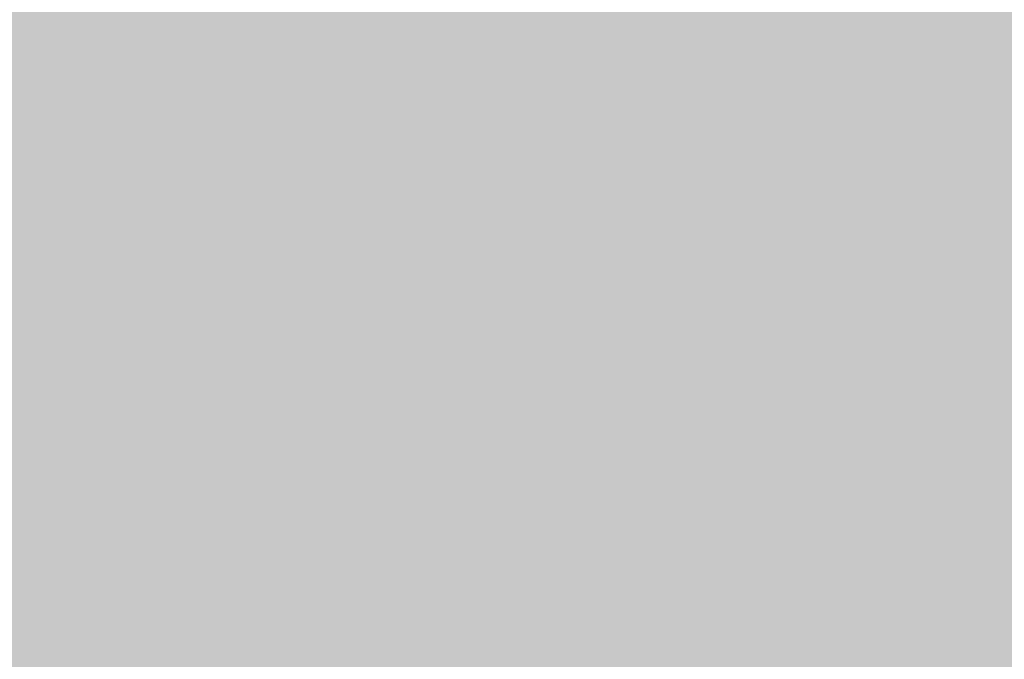
# Model space of a CAD drawing. Units: millimetres. Extents: x 0 to 2267, y 0 to 1823.
# Tile 133 of 256: x 1590 to 1632, y 1243 to 1271. Entities that reach past the tile are written whole.
import ezdxf

# ---------------------------------------------------------------- set-up
doc = ezdxf.new("R2010")
doc.units = ezdxf.units.MM
doc.header["$MEASUREMENT"] = 0
doc.layers.add('M-DIMS', color=2, linetype='Continuous', lineweight=25)
doc.layers.add('M-HATC', color=252, linetype='Continuous', lineweight=18)
doc.styles.get("Standard").update_dxf_attribs({"font": 'arial.ttf'})
doc.dimstyles.get("Standard").update_dxf_attribs({"dimtxt": 7, "dimasz": 4, "dimexe": 0.18, "dimexo": 0.0625, "dimgap": 0.09, "dimtad": 0, "dimdec": 0, "dimzin": 0, "dimdsep": 46, "dimtxsty": 'Standard', "dimcen": 0.09, "dimadec": 0, "dimazin": 0, "dimtfac": 1, "dimtdec": 0, "dimtofl": 0, "dimtmove": 0, "dimatfit": 3, "dimfxl": 1, "dimtolj": 1, "dimtzin": 0, "dimarcsym": 0})

# ---------------------------------------------------------------- blocks, each defined once
blk = doc.blocks.new('*D19')
at = {"layer": 'Defpoints', "color": 0, "transparency": 16777216}
for p in [(1605.34, 1483.304), (1445.529, 1333.885)]:
    blk.add_point(p, dxfattribs=at)
at = {"layer": 'M-DIMS', "color": 0, "lineweight": -2, "transparency": 16777216}
for p, q in [((1605.25, 1483.304), (1605.43, 1483.304)), ((1605.34, 1483.214), (1605.34, 1483.394)), ((1366.324, 1259.831), (1442.607, 1331.153))]:
    blk.add_line(p, q, dxfattribs=at)
at = {"layer": 'M-DIMS', "color": 0, "transparency": 16777216}
blk.add_solid([(1442.152, 1331.64), (1443.063, 1330.666), (1445.529, 1333.885)], dxfattribs=at)
at = {"layer": 'M-DIMS', "color": 0, "transparency": 16777216, "insert": (1349.643, 1244.233), "char_height": 7, "attachment_point": 5, "rotation": 43.0753}
blk.add_mtext('\\A1;2X R218.8', dxfattribs=at)

msp = doc.modelspace()

# ---------------------------------------------------------------- hatches: boundary and pattern name
at = {"layer": 'M-HATC'}
h = msp.add_hatch(color=256, dxfattribs=at)
h.dxf.hatch_style = 1
h.paths.add_polyline_path([(2065.771, 1618.062, 0.236068), (2055.771, 1638.062), (1381.087, 1638.062, 0.236068), (1371.087, 1618.062), (1371.087, 1603.062), (2055.771, 1603.062), (2065.771, 1603.062)])
h.paths.add_polyline_path([(2062.772, 1550.296), (2062.772, 1560.296), (1374.086, 1560.296), (1374.086, 1550.296), (1374.086, 1540.296), (1384.086, 1540.296), (1389.086, 1540.296), (2062.772, 1540.296)])
h.paths.add_polyline_path([(1930.929, 1282.766), (1505.929, 1282.766), (1587.628, 1235.597, 0.131652), (1600.128, 1232.247), (1836.73, 1232.247, 0.131652), (1849.23, 1235.597)])
h.paths.add_polyline_path([(1930.929, 1117.417), (1905.929, 1117.417), (1505.929, 1117.417), (1505.929, 1077.417), (1930.929, 1077.417)])
h = msp.add_hatch(color=256, dxfattribs=at)
h.dxf.hatch_style = 1
h.paths.add_polyline_path([(2055.771, 1603.062), (1381.087, 1603.062), (1381.087, 1598.062), (2055.771, 1598.062)])
h.paths.add_polyline_path([(2055.771, 1598.062), (1381.087, 1598.062), (1381.087, 1593.062), (2055.771, 1593.062)])
h.paths.add_polyline_path([(2051.307, 1536.761), (1385.55, 1536.761), (1385.55, 1526.761), (1387.55, 1526.761), (1388.537, 1525.053), (1385.332, 1521.233), (1385.332, 1521.223), (2050.254, 1522.749), (2048.321, 1525.053), (2049.307, 1526.761), (2051.307, 1526.761)])
edge = h.paths.add_edge_path()
edge.add_arc((1847.535, 1379.149), 135, 222.60306, 222.89085, ccw=False)
edge.add_line((1748.166, 1287.766), (1683.092, 1287.766))
edge.add_arc((1583.724, 1379.149), 135, 317.10915, 317.39694, ccw=False)
edge.add_arc((1678.969, 1290.671), 5, 222.8909, 317.1091, ccw=False)
edge.add_arc((1774.213, 1379.149), 135, 222.60306, 222.89085, ccw=False)
edge.add_line((1674.845, 1287.766), (1609.771, 1287.766))
edge.add_arc((1510.403, 1379.149), 135, 317.10915, 317.39694, ccw=False)
edge.add_arc((1605.647, 1290.671), 5, 222.8909, 317.1091, ccw=False)
edge.add_arc((1700.892, 1379.149), 135, 222.60306, 222.89085, ccw=False)
edge.add_line((1601.524, 1287.766), (1536.45, 1287.766))
edge.add_arc((1437.081, 1379.149), 135, 317.10915, 317.39694, ccw=False)
edge.add_arc((1532.326, 1290.671), 5, 222.8909, 317.1091, ccw=False)
edge.add_arc((1627.571, 1379.149), 135, 222.60306, 222.89085, ccw=False)
edge.add_line((1528.203, 1287.766), (1505.929, 1287.766))
edge.add_spline(control_points=[(1505.929, 1287.766), (1504.262, 1287.766), (1504.262, 1282.766), (1505.929, 1282.766)], knot_values=[0, 0, 0, 0, 5, 5, 5, 5], degree=3, periodic=0)
edge.add_line((1505.929, 1282.766), (1930.929, 1282.766))
edge.add_spline(control_points=[(1930.929, 1282.766), (1932.596, 1282.766), (1932.596, 1287.766), (1930.929, 1287.766)], knot_values=[0, 0, 0, 0, 5, 5, 5, 5], degree=3, periodic=0)
edge.add_line((1930.929, 1287.766), (1903.056, 1287.766))
edge.add_arc((1803.688, 1379.149), 135, 317.10915, 317.39694, ccw=False)
edge.add_arc((1898.932, 1290.671), 5, 222.8909, 317.1091, ccw=False)
edge.add_arc((1994.177, 1379.149), 135, 222.60306, 222.89085, ccw=False)
edge.add_line((1894.809, 1287.766), (1829.735, 1287.766))
edge.add_arc((1730.366, 1379.149), 135, 317.10915, 317.39694, ccw=False)
edge.add_arc((1825.611, 1290.671), 5, 222.8909, 317.1091, ccw=False)
edge.add_arc((1920.856, 1379.149), 135, 222.60306, 222.89085, ccw=False)
edge.add_line((1821.487, 1287.766), (1756.413, 1287.766))
edge.add_arc((1657.045, 1379.149), 135, 317.10915, 317.39694, ccw=False)
edge.add_arc((1752.29, 1290.671), 5, 222.8909, 317.1091, ccw=False)
edge = h.paths.add_edge_path()
edge.add_spline(control_points=[(1843.429, 1227.247), (1845.096, 1227.247), (1845.096, 1232.247), (1843.429, 1232.247)], knot_values=[0, 0, 0, 0, 5, 5, 5, 5], degree=3, periodic=0)
edge.add_line((1843.429, 1232.247), (1593.429, 1232.247))
edge.add_spline(control_points=[(1593.429, 1232.247), (1591.762, 1232.247), (1591.762, 1227.247), (1593.429, 1227.247)], knot_values=[0, 0, 0, 0, 5, 5, 5, 5], degree=3, periodic=0)
edge.add_line((1593.429, 1227.247), (1843.429, 1227.247))
h.paths.add_polyline_path([(1905.929, 1127.417), (1530.929, 1127.417, 0.414214), (1520.929, 1117.417), (1530.929, 1117.417), (1915.929, 1117.417, 0.414214)])
edge = h.paths.add_edge_path()
edge.add_arc((1397.086, 1498.408), 12.73, 90.7821, 190.8787, ccw=False)
edge.add_line((1396.912, 1511.136), (1428.01, 1511.349))
edge.add_line((1428.01, 1511.349), (1433.01, 1511.349))
edge.add_line((1433.01, 1511.349), (1434.439, 1511.349))
edge.add_arc((1419.474, 1498.08), 20, 41.561, 74.0821)
edge.add_line((1424.959, 1517.314), (1399.935, 1517.256))
edge.add_spline(control_points=[(1399.931, 1517.256), (1399.884, 1517.213), (1399.833, 1517.169), (1399.777, 1517.124)], knot_values=[11.567499, 11.567499, 11.567499, 11.567499, 11.814249, 11.814249, 11.814249, 11.814249], degree=3, periodic=0)
edge.add_spline(control_points=[(1399.633, 1517.01), (1399.583, 1516.972), (1399.531, 1516.934), (1399.476, 1516.895)], knot_values=[11.167718, 11.167718, 11.167718, 11.167718, 11.365188, 11.365188, 11.365188, 11.365188], degree=3, periodic=0)
edge.add_spline(control_points=[(1399.34, 1516.8), (1399.151, 1516.672), (1398.938, 1516.538), (1398.704, 1516.399)], knot_values=[10.376405, 10.376405, 10.376405, 10.376405, 11.00994, 11.00994, 11.00994, 11.00994], degree=3, periodic=0)
edge.add_spline(control_points=[(1398.657, 1516.372), (1398.579, 1516.326), (1398.498, 1516.28), (1398.415, 1516.233)], knot_values=[10.125175, 10.125175, 10.125175, 10.125175, 10.334406, 10.334406, 10.334406, 10.334406], degree=3, periodic=0)
edge.add_spline(control_points=[(1398.264, 1516.149), (1398.196, 1516.111), (1398.126, 1516.073), (1398.055, 1516.035)], knot_values=[9.832246, 9.832246, 9.832246, 9.832246, 9.999658, 9.999658, 9.999658, 9.999658], degree=3, periodic=0)
edge.add_spline(control_points=[(1397.999, 1516.005), (1397.731, 1515.862), (1397.446, 1515.717), (1397.147, 1515.571)], knot_values=[9.161808, 9.161808, 9.161808, 9.161808, 9.787769, 9.787769, 9.787769, 9.787769], degree=3, periodic=0)
edge.add_spline(control_points=[(1397.147, 1515.571), (1396.842, 1515.423), (1396.522, 1515.274), (1396.191, 1515.126)], knot_values=[8.524455, 8.524455, 8.524455, 8.524455, 9.161808, 9.161808, 9.161808, 9.161808], degree=3, periodic=0)
edge.add_spline(control_points=[(1396.078, 1515.076), (1395.985, 1515.035), (1395.892, 1514.994), (1395.798, 1514.953)], knot_values=[8.275193, 8.275193, 8.275193, 8.275193, 8.451726, 8.451726, 8.451726, 8.451726], degree=3, periodic=0)
edge.add_spline(control_points=[(1395.602, 1514.869), (1395.5, 1514.826), (1395.397, 1514.782), (1395.293, 1514.739)], knot_values=[7.962917, 7.962917, 7.962917, 7.962917, 8.152764, 8.152764, 8.152764, 8.152764], degree=3, periodic=0)
edge.add_spline(control_points=[(1395.212, 1514.706), (1394.828, 1514.547), (1394.435, 1514.393), (1394.036, 1514.244)], knot_values=[7.21254, 7.21254, 7.21254, 7.21254, 7.913148, 7.913148, 7.913148, 7.913148], degree=3, periodic=0)
edge.add_spline(control_points=[(1394.036, 1514.244), (1393.708, 1514.121), (1393.375, 1514.003), (1393.043, 1513.889)], knot_values=[6.633733, 6.633733, 6.633733, 6.633733, 7.21254, 7.21254, 7.21254, 7.21254], degree=3, periodic=0)
edge.add_spline(control_points=[(1392.821, 1513.815), (1392.72, 1513.781), (1392.618, 1513.748), (1392.517, 1513.715)], knot_values=[6.328796, 6.328796, 6.328796, 6.328796, 6.505493, 6.505493, 6.505493, 6.505493], degree=3, periodic=0)
edge.add_spline(control_points=[(1392.517, 1513.715), (1392.319, 1513.652), (1392.121, 1513.59), (1391.924, 1513.531)], knot_values=[5.984605, 5.984605, 5.984605, 5.984605, 6.328796, 6.328796, 6.328796, 6.328796], degree=3, periodic=0)
edge.add_spline(control_points=[(1391.792, 1513.491), (1391.312, 1513.35), (1390.838, 1513.224), (1390.378, 1513.117)], knot_values=[5.066697, 5.066697, 5.066697, 5.066697, 5.907055, 5.907055, 5.907055, 5.907055], degree=3, periodic=0)
edge.add_spline(control_points=[(1390.378, 1513.117), (1390.18, 1513.071), (1389.984, 1513.028), (1389.791, 1512.99)], knot_values=[4.70367, 4.70367, 4.70367, 4.70367, 5.066695, 5.066695, 5.066695, 5.066695], degree=3, periodic=0)
edge.add_spline(control_points=[(1389.422, 1512.92), (1389.246, 1512.889), (1389.073, 1512.862), (1388.904, 1512.838)], knot_values=[4.130571, 4.130571, 4.130571, 4.130571, 4.469816, 4.469816, 4.469816, 4.469816], degree=3, periodic=0)
edge.add_spline(control_points=[(1388.904, 1512.838), (1388.591, 1512.795), (1388.291, 1512.764), (1388.007, 1512.749)], knot_values=[3.504031, 3.504031, 3.504031, 3.504031, 4.130571, 4.130571, 4.130571, 4.130571], degree=3, periodic=0)
edge.add_spline(control_points=[(1387.936, 1512.746), (1387.854, 1512.742), (1387.773, 1512.74), (1387.694, 1512.739)], knot_values=[3.268866, 3.268866, 3.268866, 3.268866, 3.451164, 3.451164, 3.451164, 3.451164], degree=3, periodic=0)
edge.add_spline(control_points=[(1387.335, 1512.744), (1387.208, 1512.75), (1387.085, 1512.76), (1386.967, 1512.774)], knot_values=[2.670686, 2.670686, 2.670686, 2.670686, 2.984, 2.984, 2.984, 2.984], degree=3, periodic=0)
edge.add_spline(control_points=[(1386.833, 1512.792), (1386.821, 1512.794), (1386.809, 1512.796), (1386.797, 1512.798)], knot_values=[2.516981, 2.516981, 2.516981, 2.516981, 2.549528, 2.549528, 2.549528, 2.549528], degree=3, periodic=0)
edge.add_spline(control_points=[(1386.453, 1512.873), (1386.426, 1512.881), (1386.399, 1512.889), (1386.373, 1512.897)], knot_values=[2.095869, 2.095869, 2.095869, 2.095869, 2.17941, 2.17941, 2.17941, 2.17941], degree=3, periodic=0)
edge.add_spline(control_points=[(1386.069, 1513.019), (1386.063, 1513.022), (1386.058, 1513.025), (1386.052, 1513.028)], knot_values=[1.72453, 1.72453, 1.72453, 1.72453, 1.745933, 1.745933, 1.745933, 1.745933], degree=3, periodic=0)
edge.add_arc((1399.474, 1498.08), 20, 131.8243, 180)
edge.add_arc((1630.334, 1505.548), 250.971, 181.70518, 236.42798)
edge.add_arc((1605.34, 1483.304), 218.782, 238.66083, 243.34961)
edge.add_arc((1647.091, 1510.359), 262.899, 183.12984, 237.85344, ccw=False)
h.paths.add_polyline_path([(1406.537, 1391.964, 0.149382), (1491.551, 1296.442, -0.129517)], flags=17)
edge = h.paths.add_edge_path()
edge.add_arc((2037.384, 1498.08), 20, 0, 48.2659)
edge.add_spline(control_points=[(2050.697, 1513.005), (2050.651, 1512.985), (2050.603, 1512.966), (2050.554, 1512.948)], knot_values=[1.835652, 1.835652, 1.835652, 1.835652, 2.000781, 2.000781, 2.000781, 2.000781], degree=3, periodic=0)
edge.add_spline(control_points=[(2050.462, 1512.917), (2050.479, 1512.922), (2050.496, 1512.928), (2050.513, 1512.934)], knot_values=[2.045477, 2.045477, 2.045477, 2.045477, 2.101389, 2.101389, 2.101389, 2.101389], degree=3, periodic=0)
edge.add_spline(control_points=[(2050.129, 1512.834), (2050.198, 1512.847), (2050.266, 1512.862), (2050.331, 1512.879)], knot_values=[2.237629, 2.237629, 2.237629, 2.237629, 2.435841, 2.435841, 2.435841, 2.435841], degree=3, periodic=0)
edge.add_spline(control_points=[(2050.095, 1512.828), (2050.106, 1512.83), (2050.118, 1512.832), (2050.129, 1512.834)], knot_values=[2.435841, 2.435841, 2.435841, 2.435841, 2.468321, 2.468321, 2.468321, 2.468321], degree=3, periodic=0)
edge.add_spline(control_points=[(2049.784, 1512.785), (2049.855, 1512.792), (2049.924, 1512.801), (2049.992, 1512.811)], knot_values=[2.563852, 2.563852, 2.563852, 2.563852, 2.748541, 2.748541, 2.748541, 2.748541], degree=3, periodic=0)
edge.add_spline(control_points=[(2049.405, 1512.762), (2049.536, 1512.765), (2049.663, 1512.773), (2049.784, 1512.785)], knot_values=[2.748541, 2.748541, 2.748541, 2.748541, 3.064882, 3.064882, 3.064882, 3.064882], degree=3, periodic=0)
edge.add_spline(control_points=[(2049.17, 1512.76), (2049.234, 1512.759), (2049.297, 1512.759), (2049.358, 1512.761)], knot_values=[3.102309, 3.102309, 3.102309, 3.102309, 3.2503, 3.2503, 3.2503, 3.2503], degree=3, periodic=0)
edge.add_spline(control_points=[(2048.857, 1512.769), (2048.964, 1512.764), (2049.068, 1512.761), (2049.17, 1512.76)], knot_values=[3.2503, 3.2503, 3.2503, 3.2503, 3.486069, 3.486069, 3.486069, 3.486069], degree=3, periodic=0)
edge.add_spline(control_points=[(2048.692, 1512.779), (2048.373, 1512.801), (2048.035, 1512.841), (2047.682, 1512.897)], knot_values=[3.606429, 3.606429, 3.606429, 3.606429, 4.2989, 4.2989, 4.2989, 4.2989], degree=3, periodic=0)
edge.add_spline(control_points=[(2047.682, 1512.897), (2047.546, 1512.919), (2047.408, 1512.942), (2047.268, 1512.969)], knot_values=[4.2989, 4.2989, 4.2989, 4.2989, 4.565769, 4.565769, 4.565769, 4.565769], degree=3, periodic=0)
edge.add_spline(control_points=[(2047.268, 1512.969), (2047.145, 1512.991), (2047.021, 1513.016), (2046.895, 1513.042)], knot_values=[4.565769, 4.565769, 4.565769, 4.565769, 4.799971, 4.799971, 4.799971, 4.799971], degree=3, periodic=0)
edge.add_spline(control_points=[(2046.895, 1513.042), (2046.529, 1513.119), (2046.151, 1513.209), (2045.768, 1513.311)], knot_values=[4.799971, 4.799971, 4.799971, 4.799971, 5.483718, 5.483718, 5.483718, 5.483718], degree=3, periodic=0)
edge.add_spline(control_points=[(2045.768, 1513.311), (2045.372, 1513.415), (2044.97, 1513.532), (2044.566, 1513.659)], knot_values=[5.483718, 5.483718, 5.483718, 5.483718, 6.187866, 6.187866, 6.187866, 6.187866], degree=3, periodic=0)
edge.add_spline(control_points=[(2044.566, 1513.659), (2044.415, 1513.706), (2044.263, 1513.755), (2044.112, 1513.805)], knot_values=[6.187866, 6.187866, 6.187866, 6.187866, 6.451551, 6.451551, 6.451551, 6.451551], degree=3, periodic=0)
edge.add_spline(control_points=[(2044.112, 1513.805), (2043.997, 1513.843), (2043.882, 1513.881), (2043.767, 1513.92)], knot_values=[6.451551, 6.451551, 6.451551, 6.451551, 6.651434, 6.651434, 6.651434, 6.651434], degree=3, periodic=0)
edge.add_spline(control_points=[(2043.767, 1513.92), (2043.372, 1514.055), (2042.977, 1514.198), (2042.589, 1514.346)], knot_values=[6.651434, 6.651434, 6.651434, 6.651434, 7.338879, 7.338879, 7.338879, 7.338879], degree=3, periodic=0)
edge.add_spline(control_points=[(2042.589, 1514.346), (2042.164, 1514.507), (2041.746, 1514.675), (2041.341, 1514.846)], knot_values=[7.338879, 7.338879, 7.338879, 7.338879, 8.089209, 8.089209, 8.089209, 8.089209], degree=3, periodic=0)
edge.add_spline(control_points=[(2041.341, 1514.846), (2041.103, 1514.946), (2040.869, 1515.048), (2040.64, 1515.15)], knot_values=[8.089209, 8.089209, 8.089209, 8.089209, 8.529587, 8.529587, 8.529587, 8.529587], degree=3, periodic=0)
edge.add_spline(control_points=[(2040.51, 1515.209), (2040.082, 1515.402), (2039.675, 1515.597), (2039.295, 1515.789)], knot_values=[8.613818, 8.613818, 8.613818, 8.613818, 9.44571, 9.44571, 9.44571, 9.44571], degree=3, periodic=0)
edge.add_spline(control_points=[(2039.295, 1515.789), (2039.062, 1515.907), (2038.839, 1516.025), (2038.629, 1516.14)], knot_values=[9.44571, 9.44571, 9.44571, 9.44571, 9.956404, 9.956404, 9.956404, 9.956404], degree=3, periodic=0)
edge.add_spline(control_points=[(2038.629, 1516.14), (2038.519, 1516.2), (2038.412, 1516.26), (2038.309, 1516.319)], knot_values=[9.956404, 9.956404, 9.956404, 9.956404, 10.223542, 10.223542, 10.223542, 10.223542], degree=3, periodic=0)
edge.add_spline(control_points=[(2038.309, 1516.319), (2038.214, 1516.374), (2038.122, 1516.428), (2038.033, 1516.481)], knot_values=[10.223542, 10.223542, 10.223542, 10.223542, 10.47051, 10.47051, 10.47051, 10.47051], degree=3, periodic=0)
edge.add_spline(control_points=[(2038.033, 1516.481), (2037.786, 1516.63), (2037.564, 1516.773), (2037.372, 1516.909)], knot_values=[10.47051, 10.47051, 10.47051, 10.47051, 11.15767, 11.15767, 11.15767, 11.15767], degree=3, periodic=0)
edge.add_spline(control_points=[(2037.372, 1516.909), (2037.279, 1516.975), (2037.193, 1517.04), (2037.114, 1517.102)], knot_values=[11.15767, 11.15767, 11.15767, 11.15767, 11.49227, 11.49227, 11.49227, 11.49227], degree=3, periodic=0)
edge.add_spline(control_points=[(2036.856, 1517.326), (2036.915, 1517.269), (2036.981, 1517.21), (2037.056, 1517.149)], knot_values=[11.577341, 11.577341, 11.577341, 11.577341, 11.91035, 11.91035, 11.91035, 11.91035], degree=3, periodic=0)
edge.add_spline(control_points=[(2036.807, 1517.375), (2036.823, 1517.359), (2036.839, 1517.342), (2036.856, 1517.326)], knot_values=[11.91035, 11.91035, 11.91035, 11.91035, 12.007402, 12.007402, 12.007402, 12.007402], degree=3, periodic=0)
edge.add_spline(control_points=[(2036.702, 1517.494), (2036.71, 1517.483), (2036.72, 1517.472), (2036.729, 1517.461)], knot_values=[12.184155, 12.184155, 12.184155, 12.184155, 12.255409, 12.255409, 12.255409, 12.255409], degree=3, periodic=0)
edge.add_spline(control_points=[(2036.616, 1517.621), (2036.62, 1517.613), (2036.624, 1517.606), (2036.629, 1517.598)], knot_values=[12.487913, 12.487913, 12.487913, 12.487913, 12.541035, 12.541035, 12.541035, 12.541035], degree=3, periodic=0)
edge.add_spline(control_points=[(2036.563, 1517.786), (2036.564, 1517.779), (2036.564, 1517.773), (2036.565, 1517.766)], knot_values=[12.911761, 12.911761, 12.911761, 12.911761, 12.968286, 12.968286, 12.968286, 12.968286], degree=3, periodic=0)
edge.add_spline(control_points=[(2036.617, 1517.93), (2036.612, 1517.926), (2036.609, 1517.921), (2036.605, 1517.916)], knot_values=[13.382527, 13.382527, 13.382527, 13.382527, 13.433791, 13.433791, 13.433791, 13.433791], degree=3, periodic=0)
edge.add_spline(control_points=[(2036.749, 1518.017), (2036.736, 1518.012), (2036.724, 1518.006), (2036.712, 1518)], knot_values=[13.726299, 13.726299, 13.726299, 13.726299, 13.809928, 13.809928, 13.809928, 13.809928], degree=3, periodic=0)
edge.add_spline(control_points=[(2036.86, 1518.053), (2036.839, 1518.047), (2036.818, 1518.042), (2036.799, 1518.035)], knot_values=[13.910887, 13.910887, 13.910887, 13.910887, 14.02153, 14.02153, 14.02153, 14.02153], degree=3, periodic=0)
edge.add_line((2036.964, 1518.08), (2032.384, 1518.08))
edge.add_line((2032.384, 1518.08), (2027.384, 1518.08))
edge.add_line((2027.384, 1518.08), (2022.384, 1518.08))
edge.add_line((2022.384, 1518.08), (2017.384, 1518.08))
edge.add_arc((2017.384, 1498.08), 20, 90, 138.439)
edge.add_line((2002.419, 1511.349), (2003.848, 1511.349))
edge.add_line((2003.848, 1511.349), (2008.848, 1511.349))
edge.add_line((2008.848, 1511.349), (2039.772, 1511.138))
edge.add_arc((2039.772, 1498.408), 12.73, -10.8787, 90, ccw=False)
edge.add_arc((1789.767, 1510.359), 262.899, 302.14656, 356.87016, ccw=False)
edge.add_arc((1831.518, 1483.304), 218.782, 296.65039, 301.33917)
edge.add_arc((1806.524, 1505.548), 250.971, 303.57202, 358.29482)
h.paths.add_polyline_path([(2030.321, 1391.964, -0.129517), (1945.307, 1296.442, 0.149382)], flags=17)
edge = h.paths.add_edge_path()
edge.add_spline(control_points=[(2037.246, 1518.082), (2037.29, 1518.081), (2037.336, 1518.08), (2037.384, 1518.08)], knot_values=[0.000012, 0.000012, 0.000012, 0.000012, 0.144754, 0.144754, 0.144754, 0.144754], degree=3, periodic=0)
edge.add_line((2037.336, 1518.08), (2037.01, 1518.08))
edge.add_spline(control_points=[(2037.01, 1518.08), (2036.982, 1518.077), (2036.956, 1518.073), (2036.931, 1518.068)], knot_values=[14.13465, 14.13465, 14.13465, 14.13465, 14.247197, 14.247197, 14.247197, 14.247197], degree=3, periodic=0)
edge.add_spline(control_points=[(2036.931, 1518.068), (2036.928, 1518.067), (2036.924, 1518.067), (2036.921, 1518.066)], knot_values=[14.118315, 14.118315, 14.118315, 14.118315, 14.13465, 14.13465, 14.13465, 14.13465], degree=3, periodic=0)
edge.add_spline(control_points=[(2036.921, 1518.066), (2036.912, 1518.064), (2036.903, 1518.063), (2036.895, 1518.061)], knot_values=[14.078086, 14.078086, 14.078086, 14.078086, 14.118315, 14.118315, 14.118315, 14.118315], degree=3, periodic=0)
edge.add_spline(control_points=[(2036.895, 1518.061), (2036.883, 1518.058), (2036.872, 1518.056), (2036.86, 1518.053)], knot_values=[14.02153, 14.02153, 14.02153, 14.02153, 14.078086, 14.078086, 14.078086, 14.078086], degree=3, periodic=0)
edge.add_spline(control_points=[(2036.86, 1518.053), (2036.839, 1518.047), (2036.818, 1518.042), (2036.799, 1518.035)], knot_values=[13.910887, 13.910887, 13.910887, 13.910887, 14.02153, 14.02153, 14.02153, 14.02153], degree=3, periodic=0)
edge.add_spline(control_points=[(2036.799, 1518.035), (2036.798, 1518.035), (2036.797, 1518.035), (2036.797, 1518.035)], knot_values=[13.906906, 13.906906, 13.906906, 13.906906, 13.910887, 13.910887, 13.910887, 13.910887], degree=3, periodic=0)
edge.add_spline(control_points=[(2036.797, 1518.035), (2036.788, 1518.032), (2036.78, 1518.029), (2036.772, 1518.026)], knot_values=[13.857826, 13.857826, 13.857826, 13.857826, 13.906906, 13.906906, 13.906906, 13.906906], degree=3, periodic=0)
edge.add_spline(control_points=[(2036.772, 1518.026), (2036.764, 1518.023), (2036.756, 1518.02), (2036.749, 1518.017)], knot_values=[13.809928, 13.809928, 13.809928, 13.809928, 13.857826, 13.857826, 13.857826, 13.857826], degree=3, periodic=0)
edge.add_spline(control_points=[(2036.749, 1518.017), (2036.736, 1518.012), (2036.724, 1518.006), (2036.712, 1518)], knot_values=[13.726299, 13.726299, 13.726299, 13.726299, 13.809928, 13.809928, 13.809928, 13.809928], degree=3, periodic=0)
edge.add_spline(control_points=[(2036.712, 1518), (2036.712, 1518), (2036.712, 1518), (2036.711, 1518)], knot_values=[13.723993, 13.723993, 13.723993, 13.723993, 13.726299, 13.726299, 13.726299, 13.726299], degree=3, periodic=0)
edge.add_spline(control_points=[(2036.711, 1518), (2036.706, 1517.997), (2036.701, 1517.994), (2036.696, 1517.992)], knot_values=[13.686536, 13.686536, 13.686536, 13.686536, 13.723993, 13.723993, 13.723993, 13.723993], degree=3, periodic=0)
edge.add_spline(control_points=[(2036.696, 1517.992), (2036.692, 1517.989), (2036.687, 1517.987), (2036.683, 1517.984)], knot_values=[13.651251, 13.651251, 13.651251, 13.651251, 13.686536, 13.686536, 13.686536, 13.686536], degree=3, periodic=0)
edge.add_spline(control_points=[(2036.683, 1517.984), (2036.676, 1517.98), (2036.67, 1517.976), (2036.664, 1517.971)], knot_values=[13.596804, 13.596804, 13.596804, 13.596804, 13.651251, 13.651251, 13.651251, 13.651251], degree=3, periodic=0)
edge.add_spline(control_points=[(2036.664, 1517.971), (2036.664, 1517.971), (2036.663, 1517.971), (2036.663, 1517.971)], knot_values=[13.593956, 13.593956, 13.593956, 13.593956, 13.596804, 13.596804, 13.596804, 13.596804], degree=3, periodic=0)
edge.add_spline(control_points=[(2036.663, 1517.971), (2036.66, 1517.969), (2036.658, 1517.967), (2036.655, 1517.965)], knot_values=[13.570322, 13.570322, 13.570322, 13.570322, 13.593956, 13.593956, 13.593956, 13.593956], degree=3, periodic=0)
edge.add_spline(control_points=[(2036.655, 1517.965), (2036.653, 1517.963), (2036.65, 1517.961), (2036.647, 1517.959)], knot_values=[13.545477, 13.545477, 13.545477, 13.545477, 13.570322, 13.570322, 13.570322, 13.570322], degree=3, periodic=0)
edge.add_spline(control_points=[(2036.647, 1517.959), (2036.647, 1517.959), (2036.647, 1517.959), (2036.647, 1517.959)], knot_values=[13.543931, 13.543931, 13.543931, 13.543931, 13.545477, 13.545477, 13.545477, 13.545477], degree=3, periodic=0)
edge.add_spline(control_points=[(2036.647, 1517.959), (2036.641, 1517.954), (2036.636, 1517.949), (2036.631, 1517.945)], knot_values=[13.488237, 13.488237, 13.488237, 13.488237, 13.543931, 13.543931, 13.543931, 13.543931], degree=3, periodic=0)
edge.add_spline(control_points=[(2036.631, 1517.945), (2036.628, 1517.942), (2036.626, 1517.94), (2036.623, 1517.937)], knot_values=[13.460307, 13.460307, 13.460307, 13.460307, 13.488237, 13.488237, 13.488237, 13.488237], degree=3, periodic=0)
edge.add_spline(control_points=[(2036.623, 1517.937), (2036.622, 1517.936), (2036.62, 1517.934), (2036.618, 1517.932)], knot_values=[13.439712, 13.439712, 13.439712, 13.439712, 13.460307, 13.460307, 13.460307, 13.460307], degree=3, periodic=0)
edge.add_spline(control_points=[(2036.618, 1517.932), (2036.618, 1517.931), (2036.617, 1517.931), (2036.617, 1517.93)], knot_values=[13.433791, 13.433791, 13.433791, 13.433791, 13.439712, 13.439712, 13.439712, 13.439712], degree=3, periodic=0)
edge.add_spline(control_points=[(2036.617, 1517.93), (2036.612, 1517.926), (2036.609, 1517.921), (2036.605, 1517.916)], knot_values=[13.382527, 13.382527, 13.382527, 13.382527, 13.433791, 13.433791, 13.433791, 13.433791], degree=3, periodic=0)
edge.add_spline(control_points=[(2036.605, 1517.916), (2036.603, 1517.913), (2036.6, 1517.91), (2036.598, 1517.907)], knot_values=[13.350017, 13.350017, 13.350017, 13.350017, 13.382527, 13.382527, 13.382527, 13.382527], degree=3, periodic=0)
edge.add_spline(control_points=[(2036.598, 1517.907), (2036.597, 1517.906), (2036.596, 1517.904), (2036.595, 1517.903)], knot_values=[13.333922, 13.333922, 13.333922, 13.333922, 13.350017, 13.350017, 13.350017, 13.350017], degree=3, periodic=0)
edge.add_spline(control_points=[(2036.595, 1517.903), (2036.595, 1517.902), (2036.594, 1517.901), (2036.593, 1517.9)], knot_values=[13.323828, 13.323828, 13.323828, 13.323828, 13.333922, 13.333922, 13.333922, 13.333922], degree=3, periodic=0)
edge.add_spline(control_points=[(2036.593, 1517.9), (2036.59, 1517.895), (2036.588, 1517.891), (2036.585, 1517.886)], knot_values=[13.277545, 13.277545, 13.277545, 13.277545, 13.323828, 13.323828, 13.323828, 13.323828], degree=3, periodic=0)
edge.add_spline(control_points=[(2036.585, 1517.886), (2036.584, 1517.883), (2036.582, 1517.879), (2036.58, 1517.875)], knot_values=[13.240119, 13.240119, 13.240119, 13.240119, 13.277545, 13.277545, 13.277545, 13.277545], degree=3, periodic=0)
edge.add_spline(control_points=[(2036.58, 1517.875), (2036.58, 1517.874), (2036.579, 1517.873), (2036.578, 1517.872)], knot_values=[13.228211, 13.228211, 13.228211, 13.228211, 13.240119, 13.240119, 13.240119, 13.240119], degree=3, periodic=0)
edge.add_spline(control_points=[(2036.578, 1517.872), (2036.578, 1517.87), (2036.577, 1517.869), (2036.577, 1517.868)], knot_values=[13.215717, 13.215717, 13.215717, 13.215717, 13.228211, 13.228211, 13.228211, 13.228211], degree=3, periodic=0)
edge.add_spline(control_points=[(2036.577, 1517.868), (2036.575, 1517.864), (2036.574, 1517.86), (2036.573, 1517.857)], knot_values=[13.179847, 13.179847, 13.179847, 13.179847, 13.215717, 13.215717, 13.215717, 13.215717], degree=3, periodic=0)
edge.add_spline(control_points=[(2036.573, 1517.857), (2036.571, 1517.851), (2036.57, 1517.846), (2036.569, 1517.841)], knot_values=[13.132017, 13.132017, 13.132017, 13.132017, 13.179847, 13.179847, 13.179847, 13.179847], degree=3, periodic=0)
edge.add_spline(control_points=[(2036.569, 1517.841), (2036.568, 1517.84), (2036.568, 1517.839), (2036.568, 1517.838)], knot_values=[13.122482, 13.122482, 13.122482, 13.122482, 13.132017, 13.132017, 13.132017, 13.132017], degree=3, periodic=0)
edge.add_spline(control_points=[(2036.568, 1517.838), (2036.568, 1517.836), (2036.567, 1517.835), (2036.567, 1517.833)], knot_values=[13.105592, 13.105592, 13.105592, 13.105592, 13.122482, 13.122482, 13.122482, 13.122482], degree=3, periodic=0)
edge.add_spline(control_points=[(2036.567, 1517.833), (2036.566, 1517.829), (2036.566, 1517.826), (2036.565, 1517.822)], knot_values=[13.074063, 13.074063, 13.074063, 13.074063, 13.105592, 13.105592, 13.105592, 13.105592], degree=3, periodic=0)
edge.add_spline(control_points=[(2036.565, 1517.822), (2036.565, 1517.822), (2036.565, 1517.822), (2036.565, 1517.822)], knot_values=[13.074043, 13.074043, 13.074043, 13.074043, 13.074063, 13.074063, 13.074063, 13.074063], degree=3, periodic=0)
edge.add_spline(control_points=[(2036.565, 1517.822), (2036.564, 1517.816), (2036.564, 1517.811), (2036.564, 1517.805)], knot_values=[13.021884, 13.021884, 13.021884, 13.021884, 13.074043, 13.074043, 13.074043, 13.074043], degree=3, periodic=0)
edge.add_spline(control_points=[(2036.564, 1517.805), (2036.564, 1517.804), (2036.564, 1517.803), (2036.564, 1517.803)], knot_values=[13.01674, 13.01674, 13.01674, 13.01674, 13.021884, 13.021884, 13.021884, 13.021884], degree=3, periodic=0)
edge.add_spline(control_points=[(2036.564, 1517.803), (2036.563, 1517.801), (2036.563, 1517.798), (2036.563, 1517.796)], knot_values=[12.996438, 12.996438, 12.996438, 12.996438, 13.01674, 13.01674, 13.01674, 13.01674], degree=3, periodic=0)
edge.add_spline(control_points=[(2036.563, 1517.796), (2036.563, 1517.793), (2036.563, 1517.789), (2036.563, 1517.786)], knot_values=[12.968286, 12.968286, 12.968286, 12.968286, 12.996438, 12.996438, 12.996438, 12.996438], degree=3, periodic=0)
edge.add_spline(control_points=[(2036.563, 1517.786), (2036.564, 1517.779), (2036.564, 1517.773), (2036.565, 1517.766)], knot_values=[12.911761, 12.911761, 12.911761, 12.911761, 12.968286, 12.968286, 12.968286, 12.968286], degree=3, periodic=0)
edge.add_spline(control_points=[(2036.565, 1517.766), (2036.565, 1517.766), (2036.565, 1517.766), (2036.565, 1517.766)], knot_values=[12.911017, 12.911017, 12.911017, 12.911017, 12.911761, 12.911761, 12.911761, 12.911761], degree=3, periodic=0)
edge.add_spline(control_points=[(2036.565, 1517.766), (2036.565, 1517.762), (2036.566, 1517.759), (2036.566, 1517.756)], knot_values=[12.88528, 12.88528, 12.88528, 12.88528, 12.911017, 12.911017, 12.911017, 12.911017], degree=3, periodic=0)
edge.add_spline(control_points=[(2036.566, 1517.756), (2036.567, 1517.753), (2036.567, 1517.751), (2036.568, 1517.748)], knot_values=[12.862519, 12.862519, 12.862519, 12.862519, 12.88528, 12.88528, 12.88528, 12.88528], degree=3, periodic=0)
edge.add_spline(control_points=[(2036.568, 1517.748), (2036.568, 1517.747), (2036.568, 1517.747), (2036.568, 1517.746)], knot_values=[12.858885, 12.858885, 12.858885, 12.858885, 12.862519, 12.862519, 12.862519, 12.862519], degree=3, periodic=0)
edge.add_spline(control_points=[(2036.568, 1517.746), (2036.569, 1517.74), (2036.571, 1517.733), (2036.572, 1517.726)], knot_values=[12.8053, 12.8053, 12.8053, 12.8053, 12.858885, 12.858885, 12.858885, 12.858885], degree=3, periodic=0)
edge.add_spline(control_points=[(2036.572, 1517.726), (2036.573, 1517.723), (2036.574, 1517.719), (2036.576, 1517.715)], knot_values=[12.775176, 12.775176, 12.775176, 12.775176, 12.8053, 12.8053, 12.8053, 12.8053], degree=3, periodic=0)
edge.add_spline(control_points=[(2036.576, 1517.715), (2036.576, 1517.713), (2036.577, 1517.71), (2036.578, 1517.708)], knot_values=[12.756759, 12.756759, 12.756759, 12.756759, 12.775176, 12.775176, 12.775176, 12.775176], degree=3, periodic=0)
edge.add_spline(control_points=[(2036.578, 1517.708), (2036.578, 1517.707), (2036.578, 1517.706), (2036.579, 1517.705)], knot_values=[12.748742, 12.748742, 12.748742, 12.748742, 12.756759, 12.756759, 12.756759, 12.756759], degree=3, periodic=0)
edge.add_spline(control_points=[(2036.579, 1517.705), (2036.581, 1517.698), (2036.583, 1517.692), (2036.586, 1517.685)], knot_values=[12.69959, 12.69959, 12.69959, 12.69959, 12.748742, 12.748742, 12.748742, 12.748742], degree=3, periodic=0)
edge.add_spline(control_points=[(2036.586, 1517.685), (2036.588, 1517.68), (2036.59, 1517.675), (2036.592, 1517.669)], knot_values=[12.659038, 12.659038, 12.659038, 12.659038, 12.69959, 12.69959, 12.69959, 12.69959], degree=3, periodic=0)
edge.add_spline(control_points=[(2036.592, 1517.669), (2036.594, 1517.665), (2036.596, 1517.66), (2036.598, 1517.656)], knot_values=[12.626806, 12.626806, 12.626806, 12.626806, 12.659038, 12.659038, 12.659038, 12.659038], degree=3, periodic=0)
edge.add_spline(control_points=[(2036.598, 1517.656), (2036.598, 1517.655), (2036.599, 1517.654), (2036.599, 1517.653)], knot_values=[12.619394, 12.619394, 12.619394, 12.619394, 12.626806, 12.626806, 12.626806, 12.626806], degree=3, periodic=0)
edge.add_spline(control_points=[(2036.599, 1517.653), (2036.604, 1517.642), (2036.61, 1517.632), (2036.616, 1517.621)], knot_values=[12.541039, 12.541039, 12.541039, 12.541039, 12.619394, 12.619394, 12.619394, 12.619394], degree=3, periodic=0)
edge.add_spline(control_points=[(2036.616, 1517.621), (2036.616, 1517.621), (2036.616, 1517.621), (2036.616, 1517.621)], knot_values=[12.541035, 12.541035, 12.541035, 12.541035, 12.541039, 12.541039, 12.541039, 12.541039], degree=3, periodic=0)
edge.add_spline(control_points=[(2036.616, 1517.621), (2036.62, 1517.613), (2036.624, 1517.606), (2036.629, 1517.598)], knot_values=[12.487913, 12.487913, 12.487913, 12.487913, 12.541035, 12.541035, 12.541035, 12.541035], degree=3, periodic=0)
edge.add_spline(control_points=[(2036.629, 1517.598), (2036.633, 1517.592), (2036.637, 1517.585), (2036.641, 1517.579)], knot_values=[12.443982, 12.443982, 12.443982, 12.443982, 12.487913, 12.487913, 12.487913, 12.487913], degree=3, periodic=0)
edge.add_spline(control_points=[(2036.641, 1517.579), (2036.641, 1517.578), (2036.642, 1517.576), (2036.643, 1517.575)], knot_values=[12.434996, 12.434996, 12.434996, 12.434996, 12.443982, 12.443982, 12.443982, 12.443982], degree=3, periodic=0)
edge.add_spline(control_points=[(2036.643, 1517.575), (2036.653, 1517.56), (2036.664, 1517.544), (2036.676, 1517.528)], knot_values=[12.329647, 12.329647, 12.329647, 12.329647, 12.434996, 12.434996, 12.434996, 12.434996], degree=3, periodic=0)
edge.add_spline(control_points=[(2036.676, 1517.528), (2036.684, 1517.517), (2036.693, 1517.505), (2036.702, 1517.494)], knot_values=[12.255409, 12.255409, 12.255409, 12.255409, 12.329647, 12.329647, 12.329647, 12.329647], degree=3, periodic=0)
edge.add_spline(control_points=[(2036.702, 1517.494), (2036.71, 1517.483), (2036.72, 1517.472), (2036.729, 1517.461)], knot_values=[12.184155, 12.184155, 12.184155, 12.184155, 12.255409, 12.255409, 12.255409, 12.255409], degree=3, periodic=0)
edge.add_spline(control_points=[(2036.729, 1517.461), (2036.744, 1517.444), (2036.759, 1517.426), (2036.775, 1517.409)], knot_values=[12.075961, 12.075961, 12.075961, 12.075961, 12.184155, 12.184155, 12.184155, 12.184155], degree=3, periodic=0)
edge.add_spline(control_points=[(2036.775, 1517.409), (2036.776, 1517.407), (2036.777, 1517.406), (2036.778, 1517.405)], knot_values=[12.069502, 12.069502, 12.069502, 12.069502, 12.075961, 12.075961, 12.075961, 12.075961], degree=3, periodic=0)
edge.add_spline(control_points=[(2036.778, 1517.405), (2036.788, 1517.395), (2036.797, 1517.385), (2036.807, 1517.375)], knot_values=[12.007402, 12.007402, 12.007402, 12.007402, 12.069502, 12.069502, 12.069502, 12.069502], degree=3, periodic=0)
edge.add_spline(control_points=[(2036.807, 1517.375), (2036.823, 1517.359), (2036.839, 1517.342), (2036.856, 1517.326)], knot_values=[11.91035, 11.91035, 11.91035, 11.91035, 12.007402, 12.007402, 12.007402, 12.007402], degree=3, periodic=0)
edge.add_spline(control_points=[(2036.856, 1517.326), (2036.915, 1517.269), (2036.981, 1517.21), (2037.056, 1517.149)], knot_values=[11.577341, 11.577341, 11.577341, 11.577341, 11.91035, 11.91035, 11.91035, 11.91035], degree=3, periodic=0)
edge.add_spline(control_points=[(2037.056, 1517.149), (2037.075, 1517.134), (2037.094, 1517.118), (2037.114, 1517.102)], knot_values=[11.49227, 11.49227, 11.49227, 11.49227, 11.577341, 11.577341, 11.577341, 11.577341], degree=3, periodic=0)
edge.add_spline(control_points=[(2037.114, 1517.102), (2037.193, 1517.04), (2037.279, 1516.975), (2037.372, 1516.909)], knot_values=[11.15767, 11.15767, 11.15767, 11.15767, 11.49227, 11.49227, 11.49227, 11.49227], degree=3, periodic=0)
edge.add_spline(control_points=[(2037.372, 1516.909), (2037.564, 1516.773), (2037.786, 1516.63), (2038.033, 1516.481)], knot_values=[10.47051, 10.47051, 10.47051, 10.47051, 11.15767, 11.15767, 11.15767, 11.15767], degree=3, periodic=0)
edge.add_spline(control_points=[(2038.033, 1516.481), (2038.122, 1516.428), (2038.214, 1516.374), (2038.309, 1516.319)], knot_values=[10.223542, 10.223542, 10.223542, 10.223542, 10.47051, 10.47051, 10.47051, 10.47051], degree=3, periodic=0)
edge.add_spline(control_points=[(2038.309, 1516.319), (2038.412, 1516.26), (2038.519, 1516.2), (2038.629, 1516.14)], knot_values=[9.956404, 9.956404, 9.956404, 9.956404, 10.223542, 10.223542, 10.223542, 10.223542], degree=3, periodic=0)
edge.add_spline(control_points=[(2038.629, 1516.14), (2038.839, 1516.025), (2039.062, 1515.907), (2039.295, 1515.789)], knot_values=[9.44571, 9.44571, 9.44571, 9.44571, 9.956404, 9.956404, 9.956404, 9.956404], degree=3, periodic=0)
edge.add_spline(control_points=[(2039.295, 1515.789), (2039.675, 1515.597), (2040.082, 1515.402), (2040.51, 1515.209)], knot_values=[8.613818, 8.613818, 8.613818, 8.613818, 9.44571, 9.44571, 9.44571, 9.44571], degree=3, periodic=0)
edge.add_spline(control_points=[(2040.51, 1515.209), (2040.553, 1515.189), (2040.597, 1515.17), (2040.64, 1515.15)], knot_values=[8.529587, 8.529587, 8.529587, 8.529587, 8.613818, 8.613818, 8.613818, 8.613818], degree=3, periodic=0)
edge.add_spline(control_points=[(2040.64, 1515.15), (2040.869, 1515.048), (2041.103, 1514.946), (2041.341, 1514.846)], knot_values=[8.089209, 8.089209, 8.089209, 8.089209, 8.529587, 8.529587, 8.529587, 8.529587], degree=3, periodic=0)
edge.add_spline(control_points=[(2041.341, 1514.846), (2041.746, 1514.675), (2042.164, 1514.507), (2042.589, 1514.346)], knot_values=[7.338879, 7.338879, 7.338879, 7.338879, 8.089209, 8.089209, 8.089209, 8.089209], degree=3, periodic=0)
edge.add_spline(control_points=[(2042.589, 1514.346), (2042.977, 1514.198), (2043.372, 1514.055), (2043.767, 1513.92)], knot_values=[6.651434, 6.651434, 6.651434, 6.651434, 7.338879, 7.338879, 7.338879, 7.338879], degree=3, periodic=0)
edge.add_spline(control_points=[(2043.767, 1513.92), (2043.882, 1513.881), (2043.997, 1513.843), (2044.112, 1513.805)], knot_values=[6.451551, 6.451551, 6.451551, 6.451551, 6.651434, 6.651434, 6.651434, 6.651434], degree=3, periodic=0)
edge.add_spline(control_points=[(2044.112, 1513.805), (2044.263, 1513.755), (2044.415, 1513.706), (2044.566, 1513.659)], knot_values=[6.187866, 6.187866, 6.187866, 6.187866, 6.451551, 6.451551, 6.451551, 6.451551], degree=3, periodic=0)
edge.add_spline(control_points=[(2044.566, 1513.659), (2044.97, 1513.532), (2045.372, 1513.415), (2045.768, 1513.311)], knot_values=[5.483718, 5.483718, 5.483718, 5.483718, 6.187866, 6.187866, 6.187866, 6.187866], degree=3, periodic=0)
edge.add_spline(control_points=[(2045.768, 1513.311), (2046.151, 1513.209), (2046.529, 1513.119), (2046.895, 1513.042)], knot_values=[4.799971, 4.799971, 4.799971, 4.799971, 5.483718, 5.483718, 5.483718, 5.483718], degree=3, periodic=0)
edge.add_spline(control_points=[(2046.895, 1513.042), (2047.021, 1513.016), (2047.145, 1512.991), (2047.268, 1512.969)], knot_values=[4.565769, 4.565769, 4.565769, 4.565769, 4.799971, 4.799971, 4.799971, 4.799971], degree=3, periodic=0)
edge.add_spline(control_points=[(2047.268, 1512.969), (2047.408, 1512.942), (2047.546, 1512.919), (2047.682, 1512.897)], knot_values=[4.2989, 4.2989, 4.2989, 4.2989, 4.565769, 4.565769, 4.565769, 4.565769], degree=3, periodic=0)
edge.add_spline(control_points=[(2047.682, 1512.897), (2048.035, 1512.841), (2048.373, 1512.801), (2048.692, 1512.779)], knot_values=[3.606429, 3.606429, 3.606429, 3.606429, 4.2989, 4.2989, 4.2989, 4.2989], degree=3, periodic=0)
edge.add_spline(control_points=[(2048.692, 1512.779), (2048.748, 1512.775), (2048.803, 1512.772), (2048.857, 1512.769)], knot_values=[3.486069, 3.486069, 3.486069, 3.486069, 3.606429, 3.606429, 3.606429, 3.606429], degree=3, periodic=0)
edge.add_spline(control_points=[(2048.857, 1512.769), (2048.964, 1512.764), (2049.068, 1512.761), (2049.17, 1512.76)], knot_values=[3.2503, 3.2503, 3.2503, 3.2503, 3.486069, 3.486069, 3.486069, 3.486069], degree=3, periodic=0)
edge.add_spline(control_points=[(2049.17, 1512.76), (2049.234, 1512.759), (2049.297, 1512.759), (2049.358, 1512.761)], knot_values=[3.102309, 3.102309, 3.102309, 3.102309, 3.2503, 3.2503, 3.2503, 3.2503], degree=3, periodic=0)
edge.add_spline(control_points=[(2049.358, 1512.761), (2049.374, 1512.761), (2049.39, 1512.761), (2049.405, 1512.762)], knot_values=[3.064882, 3.064882, 3.064882, 3.064882, 3.102309, 3.102309, 3.102309, 3.102309], degree=3, periodic=0)
edge.add_spline(control_points=[(2049.405, 1512.762), (2049.536, 1512.765), (2049.663, 1512.773), (2049.784, 1512.785)], knot_values=[2.748541, 2.748541, 2.748541, 2.748541, 3.064882, 3.064882, 3.064882, 3.064882], degree=3, periodic=0)
edge.add_spline(control_points=[(2049.784, 1512.785), (2049.855, 1512.792), (2049.924, 1512.801), (2049.992, 1512.811)], knot_values=[2.563852, 2.563852, 2.563852, 2.563852, 2.748541, 2.748541, 2.748541, 2.748541], degree=3, periodic=0)
edge.add_spline(control_points=[(2049.992, 1512.811), (2050.026, 1512.816), (2050.061, 1512.822), (2050.095, 1512.828)], knot_values=[2.468321, 2.468321, 2.468321, 2.468321, 2.563852, 2.563852, 2.563852, 2.563852], degree=3, periodic=0)
edge.add_spline(control_points=[(2050.095, 1512.828), (2050.106, 1512.83), (2050.118, 1512.832), (2050.129, 1512.834)], knot_values=[2.435841, 2.435841, 2.435841, 2.435841, 2.468321, 2.468321, 2.468321, 2.468321], degree=3, periodic=0)
edge.add_spline(control_points=[(2050.129, 1512.834), (2050.198, 1512.847), (2050.266, 1512.862), (2050.331, 1512.879)], knot_values=[2.237629, 2.237629, 2.237629, 2.237629, 2.435841, 2.435841, 2.435841, 2.435841], degree=3, periodic=0)
edge.add_spline(control_points=[(2050.331, 1512.879), (2050.375, 1512.891), (2050.419, 1512.903), (2050.462, 1512.917)], knot_values=[2.101389, 2.101389, 2.101389, 2.101389, 2.237629, 2.237629, 2.237629, 2.237629], degree=3, periodic=0)
edge.add_spline(control_points=[(2050.462, 1512.917), (2050.479, 1512.922), (2050.496, 1512.928), (2050.513, 1512.934)], knot_values=[2.045477, 2.045477, 2.045477, 2.045477, 2.101389, 2.101389, 2.101389, 2.101389], degree=3, periodic=0)
edge.add_spline(control_points=[(2050.513, 1512.934), (2050.527, 1512.938), (2050.54, 1512.943), (2050.554, 1512.948)], knot_values=[2.000781, 2.000781, 2.000781, 2.000781, 2.045477, 2.045477, 2.045477, 2.045477], degree=3, periodic=0)
edge.add_spline(control_points=[(2050.554, 1512.948), (2050.603, 1512.966), (2050.651, 1512.985), (2050.697, 1513.005)], knot_values=[1.835652, 1.835652, 1.835652, 1.835652, 2.000781, 2.000781, 2.000781, 2.000781], degree=3, periodic=0)
edge.add_arc((2037.384, 1498.08), 20, 48.2659, 90.1299)
edge = h.paths.add_edge_path(flags=16)
edge.add_spline(control_points=[(1386.139, 1512.986), (1388.92, 1511.739), (1398.039, 1515.519), (1399.931, 1517.256)], knot_values=[1.831046, 1.831046, 1.831046, 1.831046, 11.814249, 11.814249, 11.814249, 11.814249], degree=3, periodic=0)
edge.add_line((1399.931, 1517.256), (1393.743, 1517.242))
edge.add_arc((1399.474, 1498.08), 20, 106.6501, 131.8173)

# ---------------------------------------------------------------- dimensions: what is measured, and where the dimension line sits
at = {"layer": 'M-DIMS'}
dim = msp.add_radius_dim(center=(1605.34, 1483.304), mpoint=(1445.529, 1333.885), text='2X <>', dimstyle='Standard', override={"dimdec": 1, "dimlfac": 1, "dimrnd": 0, "dimzin": 0, "dimdsep": 46, "dimlunit": 2}, dxfattribs=at)
dim.commit()
dim.dimension.update_dxf_attribs({"geometry": '*D19', "text_midpoint": (1349.643, 1244.233), "dimtype": 164})

doc.saveas('drawing.dxf')
